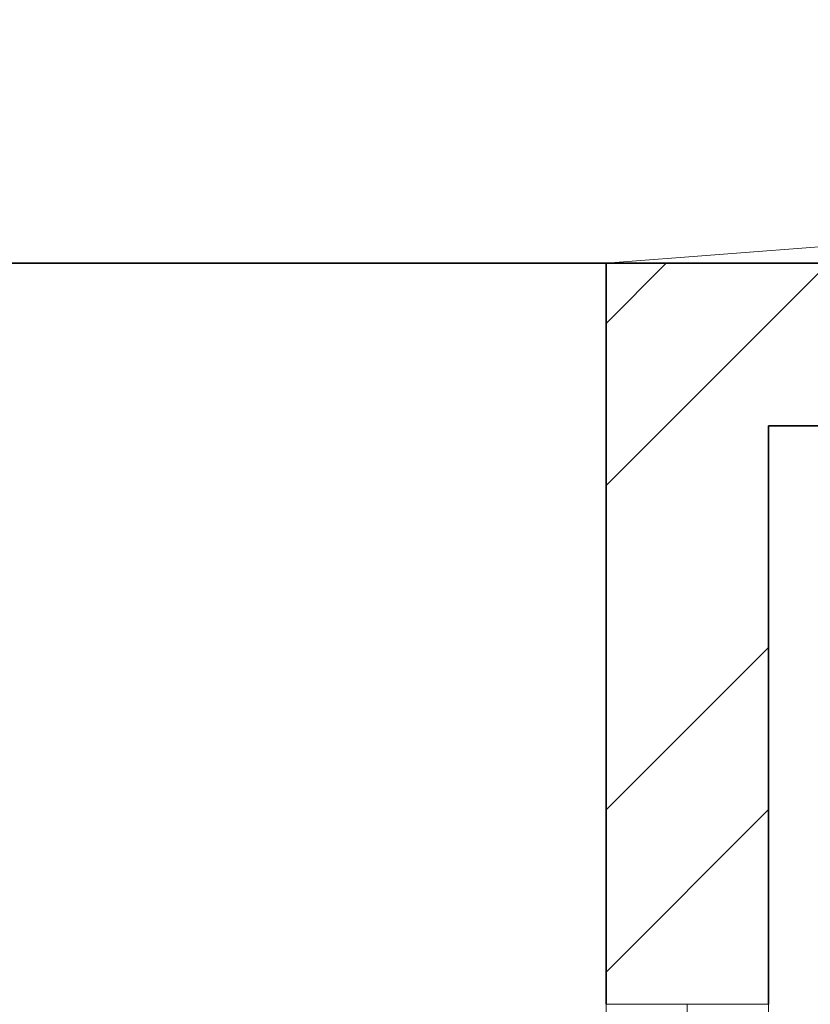
# Model space of a CAD drawing. Units: inches. Extents: x 1885 to 2748, y 783 to 2421.
# Tile 33 of 117: x 1991 to 2013, y 1503 to 1531. Entities that reach past the tile are written whole.
import ezdxf

# ---------------------------------------------------------------- set-up
doc = ezdxf.new("R2010")
doc.units = ezdxf.units.IN
for name, color, linetype, lineweight in [('A-FLOR-OPEN', 8, 'Continuous', 13), ('A-GLAZ', 181, 'Continuous', 18), ('A-WALL', 7, 'Continuous', 35)]:
    doc.layers.add(name, color=color, linetype=linetype, lineweight=lineweight)
doc.layers.add('A-WALL-PATT', color=85, linetype='Continuous', lineweight=13, true_color=0x58ba48)

# ---------------------------------------------------------------- blocks, each defined once
blk = doc.blocks.new('WIN-60-ALT')
for p, q in [((0.004, 59.998), (4.504, 59.998)), ((0.004, 59.998), (0.004, -0.002)), ((4.504, 59.998), (2.254, 59.998)), ((2.254, 59.998), (2.254, -0.002)), ((4.504, -0.002), (4.504, 59.998))]:
    blk.add_line(p, q)

msp = doc.modelspace()

# ---------------------------------------------------------------- hatches: boundary and pattern name
at = {"layer": 'A-WALL-PATT'}
h = msp.add_hatch(dxfattribs=at)
h.set_pattern_fill('ANSI32', color=256)
h.paths.add_polyline_path([(2007.772, 2318.006), (1980.774, 2318.006), (1980.774, 2281.215), (1985.274, 2281.215), (1985.274, 2313.506), (2007.772, 2313.506), (2007.772, 2315.756)])
h.paths.add_polyline_path([(2094.324, 2318.006), (2067.772, 2318.006), (2067.772, 2313.506), (2094.324, 2313.506), (2094.324, 2315.756)])
h.paths.add_polyline_path([(2131.367, 2315.756), (2131.367, 2318.006), (2131.189, 2318.006), (2112.609, 2318.006), (2112.609, 2313.506), (2117.274, 2313.506), (2117.274, 2255.201), (2121.774, 2255.201), (2121.774, 2313.506), (2131.367, 2313.506)])
h.paths.add_polyline_path([(2190.512, 2318.006), (2155.367, 2318.006), (2155.367, 2313.506), (2169.774, 2313.506), (2169.774, 2229.506), (2121.774, 2229.506), (2121.774, 2233.451), (2119.524, 2233.451), (2117.274, 2233.451), (2117.274, 2201.101), (2121.774, 2201.101), (2121.774, 2225.006), (2169.774, 2225.006), (2169.774, 2165.006), (2306.274, 2165.006), (2306.274, 2066.006), (2310.774, 2066.006), (2344.274, 2066.006), (2486.274, 2066.006), (2486.274, 1886.006), (2483.02, 1886.006), (2483.02, 1881.506), (2486.274, 1881.506), (2486.274, 1880.678), (2490.774, 1880.678), (2490.774, 2070.506), (2344.274, 2070.506), (2310.774, 2070.506), (2310.774, 2165.006), (2310.774, 2173.636), (2308.524, 2173.636), (2306.274, 2173.636), (2306.274, 2169.506), (2174.274, 2169.506), (2174.274, 2313.506), (2190.512, 2313.506), (2190.512, 2315.756)])
h.paths.add_polyline_path([(1985.274, 2221.215), (1980.774, 2221.215), (1980.774, 2165.006), (1992.774, 2165.006), (1992.774, 2141.927), (1997.274, 2141.927), (1997.274, 2165.006), (2117.274, 2165.006), (2117.274, 2163.126), (2121.774, 2163.126), (2121.774, 2172.734), (2119.524, 2172.734), (2117.274, 2172.734), (2117.274, 2169.506), (1985.274, 2169.506)])
h.paths.add_polyline_path([(1997.274, 2105.927), (1992.774, 2105.927), (1992.774, 2070.506), (2016.774, 2070.506), (2016.774, 2059.123), (2019.024, 2059.123), (2021.274, 2059.123), (2021.274, 2070.506), (2117.274, 2070.506), (2117.274, 2022.506), (2114.423, 2022.506), (2114.423, 2018.006), (2123.627, 2018.006), (2123.627, 2020.256), (2123.627, 2022.506), (2121.774, 2022.506), (2121.774, 2142.587), (2119.524, 2142.587), (2117.274, 2142.587), (2117.274, 2075.006), (1997.274, 2075.006)])
h.paths.add_polyline_path([(2092.029, 2020.256), (2092.029, 2022.506), (2021.274, 2022.506), (2021.274, 2035.123), (2016.774, 2035.123), (2016.774, 2018.006), (2016.774, 1978.784), (2021.274, 1978.784), (2021.274, 2018.006), (2092.029, 2018.006)])
h.paths.add_polyline_path([(2260.938, 2022.506), (2153.105, 2022.506), (2153.105, 2020.256), (2153.105, 2018.006), (2155.274, 2018.006), (2155.274, 1886.006), (2107.629, 1886.006), (2107.629, 1881.506), (2182.911, 1881.506), (2182.911, 1883.756), (2182.911, 1886.006), (2159.774, 1886.006), (2159.774, 2018.006), (2260.938, 2018.006), (2260.938, 2020.256)])
h.paths.add_polyline_path([(2047.629, 1883.756), (2047.629, 1886.006), (2021.274, 1886.006), (2021.274, 1918.784), (2019.024, 1918.784), (2016.774, 1918.784), (2016.774, 1881.506), (2047.629, 1881.506)])
h.paths.add_polyline_path([(2306.361, 1883.756), (2306.361, 1886.006), (2296.274, 1886.006), (2296.274, 1982.006), (2316.535, 1982.006), (2316.535, 1984.256), (2316.535, 1986.506), (2296.274, 1986.506), (2296.274, 2022.506), (2289.276, 2022.506), (2289.276, 2018.006), (2291.774, 2018.006), (2291.774, 1886.006), (2242.911, 1886.006), (2242.911, 1881.506), (2306.361, 1881.506)], flags=17)
h.paths.add_polyline_path([(1985.274, 1843.006), (2021.6, 1843.006), (2021.534, 1845.441), (2021.477, 1847.506), (1980.774, 1847.506), (1980.774, 1809.446), (1985.274, 1809.446)])
h.paths.add_polyline_path([(2131.482, 1845.256), (2131.482, 1847.506), (2081.534, 1847.506), (2081.534, 1843.006), (2117.274, 1843.006), (2117.274, 1784.147), (2119.524, 1784.147), (2121.774, 1784.147), (2121.774, 1843.006), (2131.482, 1843.006)])
h.paths.add_polyline_path([(2203.886, 1847.506), (2155.482, 1847.506), (2155.482, 1843.006), (2169.774, 1843.006), (2169.774, 1759.006), (2121.774, 1759.006), (2121.774, 1761.457), (2117.274, 1761.457), (2117.274, 1730.429), (2121.774, 1730.429), (2121.774, 1754.506), (2177.421, 1754.506), (2177.421, 1756.756), (2177.421, 1759.006), (2174.274, 1759.006), (2174.274, 1843.006), (2203.886, 1843.006)])
h.paths.add_polyline_path([(2335.554, 1845.256), (2335.554, 1847.506), (2239.886, 1847.506), (2239.886, 1843.006), (2306.274, 1843.006), (2306.274, 1759.006), (2199.486, 1759.006), (2199.486, 1754.506), (2310.774, 1754.506), (2310.774, 1843.006), (2335.554, 1843.006)])
h.paths.add_polyline_path([(2348.774, 2022.506), (2344.274, 2022.506), (2344.274, 1986.506), (2341.681, 1986.506), (2341.681, 1982.006), (2344.274, 1982.006), (2344.274, 1886.006), (2330.361, 1886.006), (2330.361, 1881.506), (2361.627, 1881.506), (2361.627, 1883.756), (2361.627, 1886.006), (2348.774, 1886.006)], flags=17)
h.paths.add_polyline_path([(2283.251, 2315.756), (2283.251, 2318.006), (2238.512, 2318.006), (2238.512, 2313.506), (2283.251, 2313.506)], flags=17)
h.paths.add_polyline_path([(2363.274, 2348.006), (2388.677, 2348.006), (2388.677, 2350.256), (2388.677, 2352.506), (2358.774, 2352.506), (2358.774, 2348.006), (2358.774, 2318.006), (2344.481, 2318.006), (2344.481, 2313.506), (2358.774, 2313.506), (2358.774, 2229.506), (2310.774, 2229.506), (2310.774, 2231.952), (2306.274, 2231.952), (2306.274, 2205.611), (2310.774, 2205.611), (2310.774, 2225.006), (2358.774, 2225.006), (2358.774, 2211.506), (2452.329, 2211.506), (2452.329, 2213.756), (2452.329, 2216.006), (2363.274, 2216.006), (2363.274, 2318.006)])
h.paths.add_polyline_path([(2310.774, 2313.506), (2320.481, 2313.506), (2320.481, 2315.756), (2320.481, 2318.006), (2302.728, 2318.006), (2302.728, 2313.506), (2306.274, 2313.506), (2306.274, 2251.076), (2310.774, 2251.076)], flags=17)
h.paths.add_polyline_path([(2490.774, 2352.506), (2486.274, 2352.506), (2448.677, 2352.506), (2448.677, 2348.006), (2486.274, 2348.006), (2486.274, 2318.006), (2486.274, 2216.006), (2481.78, 2216.006), (2481.78, 2211.506), (2486.274, 2211.506), (2486.274, 2165.006), (2493.289, 2165.006), (2493.289, 2167.256), (2493.289, 2169.506), (2490.774, 2169.506), (2490.774, 2313.506), (2494.429, 2313.506), (2494.429, 2318.006), (2490.774, 2318.006)])
h.paths.add_polyline_path([(2534.653, 2318.006), (2515.691, 2318.006), (2515.691, 2313.506), (2534.653, 2313.506), (2534.653, 2315.756)])
h.paths.add_polyline_path([(2618.274, 2318.006), (2594.653, 2318.006), (2594.653, 2313.506), (2613.774, 2313.506), (2613.774, 2281.706), (2618.274, 2281.706)])
h.paths.add_polyline_path([(2618.274, 2221.706), (2613.774, 2221.706), (2613.774, 2169.506), (2554.019, 2169.506), (2554.019, 2165.006), (2613.774, 2165.006), (2613.774, 2152.878), (2618.274, 2152.878)])
h.paths.add_polyline_path([(2618.274, 2128.878), (2616.024, 2128.878), (2613.774, 2128.878), (2613.774, 2117.006), (2529.774, 2117.006), (2529.774, 2165.006), (2532.848, 2165.006), (2532.848, 2169.506), (2522.867, 2169.506), (2522.867, 2165.006), (2525.274, 2165.006), (2525.274, 2117.006), (2525.274, 2112.506), (2525.274, 2108.576), (2529.774, 2108.576), (2529.774, 2112.506), (2613.774, 2112.506), (2613.774, 2080.19), (2618.274, 2080.19)])
h.paths.add_polyline_path([(2618.274, 2044.19), (2616.024, 2044.19), (2613.774, 2044.19), (2613.774, 2015.506), (2529.774, 2015.506), (2529.774, 2088.582), (2527.524, 2088.582), (2525.274, 2088.582), (2525.274, 2011.006), (2613.774, 2011.006), (2613.774, 1956.755), (2618.274, 1956.755)])
h.paths.add_polyline_path([(2618.274, 1881.506), (2618.274, 1896.755), (2613.774, 1896.755), (2613.774, 1881.506), (2613.774, 1847.506), (2592.715, 1847.506), (2592.715, 1843.006), (2613.774, 1843.006), (2613.774, 1765.006), (2613.774, 1760.506), (2609.621, 1760.506), (2609.621, 1756.006), (2613.774, 1756.006), (2613.774, 1660.006), (2608.544, 1660.006), (2608.544, 1655.506), (2613.774, 1655.506), (2613.774, 1508.158), (2618.274, 1508.158)])
h.paths.add_polyline_path([(2565.774, 1843.006), (2568.997, 1843.006), (2568.997, 1847.506), (2490.774, 1847.506), (2490.774, 1849.7), (2488.524, 1849.7), (2486.274, 1849.7), (2486.274, 1847.506), (2477.274, 1847.506), (2477.274, 1838.506), (2477.274, 1821.493), (2486.274, 1821.493), (2486.274, 1838.506), (2561.274, 1838.506), (2561.274, 1765.006), (2486.274, 1765.006), (2486.274, 1786.157), (2477.274, 1786.157), (2477.274, 1765.006), (2477.274, 1756.006), (2486.274, 1756.006), (2565.774, 1756.006), (2585.621, 1756.006), (2585.621, 1758.256), (2585.621, 1760.506), (2565.774, 1760.506), (2565.774, 1765.006)])
h.paths.add_polyline_path([(2486.274, 1651.006), (2561.274, 1651.006), (2561.274, 1567.006), (2486.274, 1567.006), (2486.274, 1591.321), (2477.274, 1591.321), (2477.274, 1567.006), (2477.274, 1558.006), (2477.274, 1555.439), (2481.774, 1555.439), (2481.774, 1558.006), (2568.653, 1558.006), (2568.653, 1560.256), (2568.653, 1562.506), (2565.774, 1562.506), (2565.774, 1655.506), (2584.544, 1655.506), (2584.544, 1657.756), (2584.544, 1660.006), (2565.774, 1660.006), (2486.274, 1660.006), (2477.274, 1660.006), (2477.274, 1651.006), (2477.274, 1632.989), (2486.274, 1632.989)])
h.paths.add_polyline_path([(2449.967, 1883.756), (2449.967, 1886.006), (2421.627, 1886.006), (2421.627, 1881.506), (2449.967, 1881.506)], flags=17)
h.paths.add_polyline_path([(2447.274, 1847.506), (2395.554, 1847.506), (2395.554, 1843.006), (2442.774, 1843.006), (2442.774, 1809.27), (2447.274, 1809.27)])
h.paths.add_polyline_path([(1985.274, 1749.446), (1980.774, 1749.446), (1980.774, 1694.504), (1985.274, 1694.504), (1985.274, 1694.506), (1986.897, 1694.506), (1986.897, 1697.78), (1986.897, 1699.006), (1985.274, 1699.006)])
h.paths.add_polyline_path([(2152.774, 1699.006), (2121.774, 1699.006), (2121.774, 1703.668), (2119.524, 1703.668), (2117.274, 1703.668), (2117.274, 1699.006), (2009.219, 1699.006), (2009.219, 1694.506), (2148.274, 1694.506), (2148.274, 1692.631), (2152.774, 1692.631)])
h.paths.add_polyline_path([(2016.274, 1694.506), (2011.774, 1694.506), (2011.774, 1558.006), (2040.806, 1558.006), (2040.806, 1560.256), (2040.806, 1562.506), (2016.274, 1562.506)])
h.paths.add_polyline_path([(2152.774, 1663.017), (2150.524, 1663.017), (2148.274, 1663.017), (2148.274, 1562.506), (2100.806, 1562.506), (2100.806, 1558.006), (2165.119, 1558.006), (2165.119, 1560.256), (2165.119, 1562.506), (2152.774, 1562.506), (2152.774, 1610.506), (2224.774, 1610.506), (2224.774, 1607.99), (2229.274, 1607.99), (2229.274, 1615.006), (2152.774, 1615.006)])
h.paths.add_polyline_path([(2238.613, 1560.256), (2238.613, 1562.506), (2229.274, 1562.506), (2229.274, 1588.756), (2227.024, 1588.763), (2224.774, 1588.771), (2224.774, 1562.506), (2189.119, 1562.506), (2189.119, 1558.006), (2238.613, 1558.006)])
h.paths.add_polyline_path([(2336.024, 1560.256), (2336.024, 1562.506), (2310.774, 1562.506), (2310.774, 1656.347), (2308.524, 1656.347), (2306.274, 1656.347), (2306.274, 1562.506), (2286.613, 1562.506), (2286.613, 1558.006), (2336.024, 1558.006)])
h.paths.add_polyline_path([(2447.274, 1690.968), (2445.024, 1690.968), (2442.774, 1690.968), (2442.774, 1687.006), (2306.274, 1687.006), (2306.274, 1680.75), (2310.774, 1680.75), (2310.774, 1682.506), (2442.774, 1682.506), (2442.774, 1562.506), (2396.024, 1562.506), (2396.024, 1558.006), (2447.274, 1558.006)])
h.paths.add_polyline_path([(2447.274, 1749.27), (2445.024, 1749.27), (2442.774, 1749.27), (2442.774, 1717.232), (2447.274, 1717.232)])
h.paths.add_polyline_path([(2044.674, 1521.756), (2044.674, 1524.006), (2007.274, 1524.006), (2007.274, 1503.49), (2009.524, 1503.49), (2011.774, 1503.49), (2011.774, 1519.506), (2044.674, 1519.506)])
h.paths.add_polyline_path([(2177.969, 1521.756), (2177.969, 1524.006), (2104.674, 1524.006), (2104.674, 1519.506), (2145.774, 1519.506), (2145.774, 1387.506), (2143.37, 1387.506), (2143.37, 1383.006), (2251.585, 1383.006), (2251.585, 1385.256), (2251.585, 1387.506), (2150.274, 1387.506), (2150.274, 1519.506), (2177.969, 1519.506)])
h.paths.add_polyline_path([(2298.704, 1524.006), (2237.969, 1524.006), (2237.969, 1519.506), (2282.274, 1519.506), (2282.274, 1387.506), (2279.683, 1387.506), (2279.683, 1383.006), (2286.774, 1383.006), (2286.774, 1419.006), (2312.451, 1419.006), (2312.451, 1421.256), (2312.451, 1423.506), (2286.774, 1423.506), (2286.774, 1519.506), (2298.704, 1519.506), (2298.704, 1521.722)], flags=17)
h.paths.add_polyline_path([(2361.897, 1521.756), (2361.897, 1524.006), (2322.704, 1524.006), (2322.704, 1519.506), (2334.774, 1519.506), (2334.774, 1423.506), (2331.93, 1423.506), (2331.93, 1419.006), (2334.774, 1419.006), (2334.774, 1387.506), (2334.774, 1383.228), (2339.274, 1383.228), (2339.274, 1387.506), (2339.274, 1519.506), (2361.897, 1519.506)], flags=17)
h.paths.add_polyline_path([(2447.274, 1521.756), (2447.274, 1524.006), (2421.897, 1524.006), (2421.897, 1519.506), (2447.274, 1519.506)], flags=17)
h.paths.add_polyline_path([(2481.774, 1529.6), (2479.524, 1529.6), (2477.274, 1529.6), (2477.274, 1524.006), (2474.489, 1524.006), (2474.489, 1519.506), (2477.274, 1519.506), (2477.274, 1334.506), (2296.774, 1334.506), (2296.774, 1240.506), (2160.274, 1240.506), (2160.274, 1180.506), (2112.274, 1180.506), (2112.274, 1207.692), (2110.024, 1207.692), (2107.774, 1207.692), (2107.774, 1171.609), (2112.274, 1171.609), (2112.274, 1176.006), (2160.274, 1176.006), (2160.274, 1092.006), (2144.221, 1092.006), (2144.221, 1087.506), (2189.497, 1087.506), (2189.497, 1089.756), (2189.497, 1092.006), (2164.774, 1092.006), (2164.774, 1236.006), (2296.774, 1236.006), (2296.774, 1231.912), (2301.274, 1231.912), (2301.274, 1330.006), (2481.774, 1330.006), (2481.774, 1387.506)])
h.paths.add_polyline_path([(2618.274, 1448.158), (2613.774, 1448.158), (2613.774, 1382.506), (2529.774, 1382.506), (2525.274, 1382.506), (2525.274, 1307.062), (2529.774, 1307.062), (2529.774, 1378.006), (2613.774, 1378.006), (2613.774, 1354.988), (2618.274, 1354.988)])
h.paths.add_polyline_path([(2618.274, 1318.988), (2613.774, 1318.988), (2613.774, 1281.006), (2529.774, 1281.006), (2529.774, 1283.786), (2527.524, 1283.786), (2525.274, 1283.786), (2525.274, 1228.506), (2516.794, 1228.506), (2516.794, 1224.006), (2533.484, 1224.006), (2533.484, 1226.256), (2533.484, 1228.506), (2529.774, 1228.506), (2529.774, 1276.506), (2613.774, 1276.506), (2613.774, 1266.02), (2618.274, 1266.02)])
h.paths.add_polyline_path([(2618.274, 1134.964), (2613.774, 1134.964), (2613.774, 1092.006), (2594.545, 1092.006), (2594.545, 1087.506), (2618.274, 1087.506)])
h.paths.add_polyline_path([(2534.545, 1092.006), (2509.765, 1092.006), (2509.765, 1087.506), (2534.545, 1087.506), (2534.545, 1089.756)])
h.paths.add_polyline_path([(2481.274, 1224.006), (2484.117, 1224.006), (2484.117, 1226.256), (2484.117, 1228.506), (2476.774, 1228.506), (2476.774, 1198.506), (2471.61, 1198.506), (2471.61, 1194.006), (2476.774, 1194.006), (2476.774, 1062.006), (2436.894, 1062.006), (2436.894, 1057.506), (2476.774, 1057.506), (2481.274, 1057.506), (2481.274, 1062.006), (2481.274, 1087.506), (2485.354, 1087.506), (2485.354, 1089.756), (2485.354, 1092.006), (2481.274, 1092.006), (2481.274, 1117.506)])
h.paths.add_polyline_path([(2439.898, 1198.506), (2349.274, 1198.506), (2349.274, 1194.006), (2349.274, 1180.506), (2301.274, 1180.506), (2301.274, 1201.896), (2299.024, 1201.896), (2296.774, 1201.896), (2296.774, 1172.335), (2299.024, 1172.335), (2301.274, 1172.335), (2301.274, 1176.006), (2349.274, 1176.006), (2349.274, 1092.006), (2334.452, 1092.006), (2334.452, 1087.506), (2349.274, 1087.506), (2349.274, 1057.506), (2353.774, 1057.506), (2376.894, 1057.506), (2376.894, 1059.756), (2376.894, 1062.006), (2353.774, 1062.006), (2353.774, 1087.506), (2353.774, 1180.506), (2353.774, 1194.006), (2439.898, 1194.006), (2439.898, 1196.256)])
h.paths.add_polyline_path([(2270.596, 1089.756), (2270.596, 1092.006), (2249.497, 1092.006), (2249.497, 1087.506), (2270.596, 1087.506)], flags=17)
h.paths.add_polyline_path([(2310.452, 1092.006), (2301.274, 1092.006), (2301.274, 1153.292), (2296.774, 1153.292), (2296.774, 1092.006), (2293.786, 1092.006), (2293.786, 1087.506), (2310.452, 1087.506), (2310.452, 1089.756)], flags=17)
h.paths.add_polyline_path([(2112.274, 1150.328), (2110.024, 1150.328), (2107.774, 1150.328), (2107.774, 1092.006), (2104.465, 1092.006), (2104.465, 1087.506), (2120.221, 1087.506), (2120.221, 1089.756), (2120.221, 1092.006), (2112.274, 1092.006)])
h.paths.add_polyline_path([(2082.172, 1092.006), (2058.144, 1092.006), (2058.144, 1087.506), (2082.172, 1087.506), (2082.172, 1089.756)])
h.paths.add_polyline_path([(1975.774, 1145.638), (1971.274, 1145.638), (1971.274, 1087.506), (1980.774, 1087.506), (1998.144, 1087.506), (1998.144, 1089.756), (1998.144, 1092.006), (1985.274, 1092.006), (1975.774, 1092.006)])
h.paths.add_polyline_path([(2112.274, 1244.385), (2110.024, 1244.385), (2107.774, 1244.385), (2107.774, 1240.506), (1992.274, 1240.506), (1992.274, 1271.008), (1987.774, 1271.008), (1987.774, 1240.506), (1980.774, 1240.506), (1975.774, 1240.506), (1971.274, 1240.506), (1971.274, 1205.638), (1975.774, 1205.638), (1975.774, 1236.006), (2107.774, 1236.006), (2107.774, 1233.444), (2112.274, 1233.444), (2112.274, 1236.006)])
h.paths.add_polyline_path([(2112.274, 1383.006), (2114.783, 1383.006), (2114.783, 1385.256), (2114.783, 1387.506), (2102.476, 1387.506), (2102.476, 1383.006), (2107.774, 1383.006), (2107.774, 1335.006), (2011.774, 1335.006), (2011.774, 1349.939), (2007.274, 1349.939), (2007.274, 1335.006), (1987.774, 1335.006), (1987.774, 1330.506), (1987.774, 1307.008), (1992.274, 1307.008), (1992.274, 1330.506), (2007.274, 1330.506), (2107.774, 1330.506), (2107.774, 1264.711), (2112.274, 1264.711)])
h.paths.add_polyline_path([(2077.857, 1387.506), (2011.774, 1387.506), (2011.774, 1390.036), (2009.524, 1390.036), (2007.274, 1390.036), (2007.274, 1373.939), (2011.774, 1373.939), (2011.774, 1383.006), (2077.857, 1383.006)])
h.paths.add_polyline_path([(2011.774, 1443.49), (2007.274, 1443.49), (2007.274, 1410.248), (2011.774, 1410.248)])

# ---------------------------------------------------------------- linework, layer by layer
at = {"layer": 'A-FLOR-OPEN'}
msp.add_line((2007.274, 1524.006), (2447.274, 1558.006), dxfattribs=at)
at = {"layer": 'A-WALL'}
for p, q in [((1980.774, 1524.006), (2044.674, 1524.006)), ((2007.274, 1503.49), (2007.274, 1524.006)), ((2011.774, 1519.506), (2011.774, 1503.49)), ((2011.774, 1519.506), (2044.674, 1519.506))]:
    msp.add_line(p, q, dxfattribs=at)

# ---------------------------------------------------------------- block references
at = {"layer": 'A-GLAZ', "extrusion": (0, 0, -1), "zscale": -1}
msp.add_blockref('WIN-60-ALT', (-2011.777, 1443.493), dxfattribs=at)

doc.saveas('drawing.dxf')
